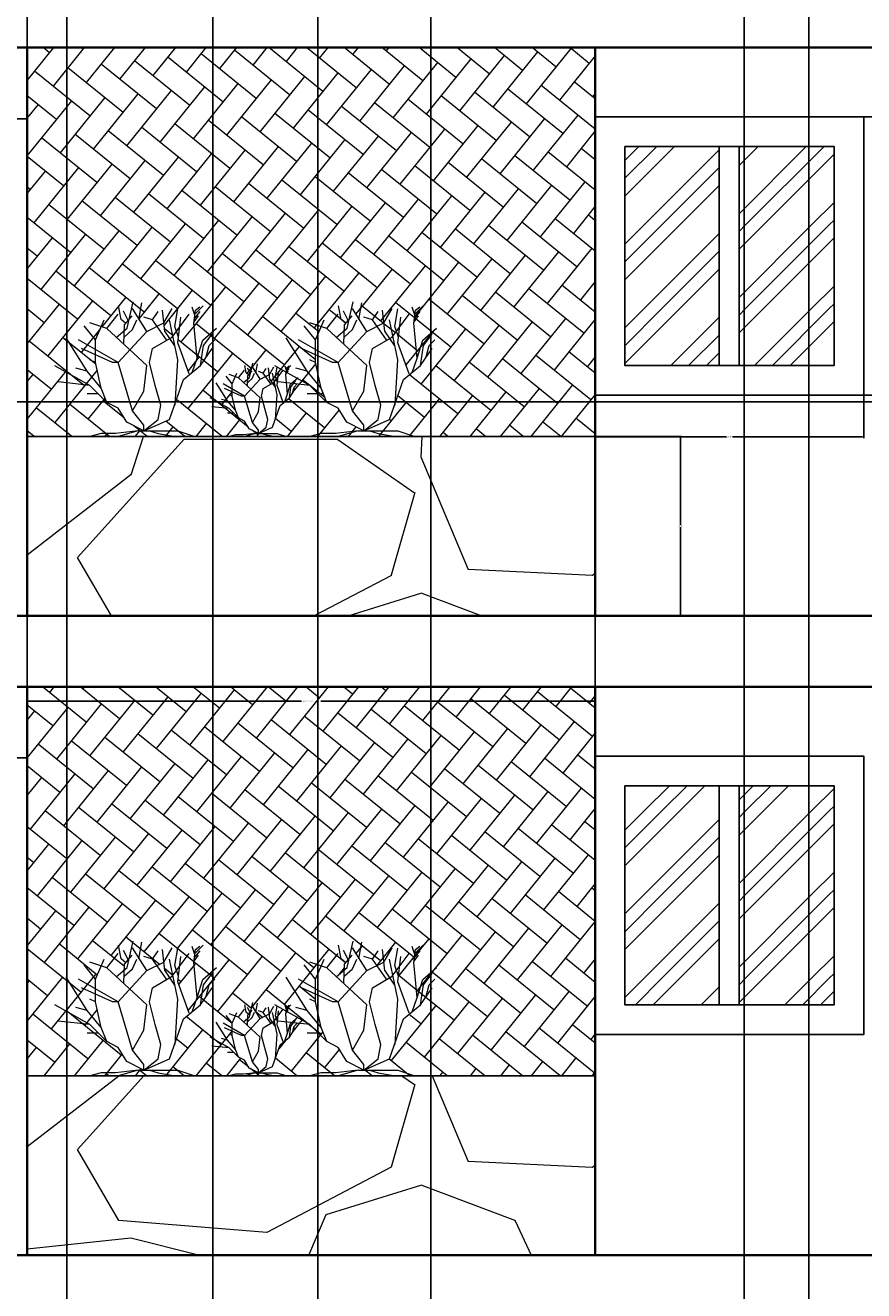
# Model space of a CAD drawing. Units: inches. Extents: x -8 to 554, y -200 to 499.
# Tile 9 of 12: x 216 to 358, y 121 to 335. Entities that reach past the tile are written whole.
import ezdxf

# ---------------------------------------------------------------- set-up
doc = ezdxf.new("R2010")
doc.units = ezdxf.units.IN
doc.header["$MEASUREMENT"] = 0
for name, color, linetype, lineweight in [('A-ANNO-DIMS', 2, 'Continuous', 18), ('A-DOOR', 3, 'Continuous', 25), ('A-FLOR', 7, 'Continuous', 35), ('A-GLAZ', 4, 'Continuous', 25), ('A-GLAZ-PATT', 252, 'Continuous', 13), ('A-WALL', 7, 'Continuous', 35), ('A-WALL-PATT', 252, 'Continuous', 13), ('A-WALL-PRPT', 7, 'Continuous', 25), ('L-PLNT-TREE', 94, 'Continuous', 13)]:
    doc.layers.add(name, color=color, linetype=linetype, lineweight=lineweight)
doc.styles.get("Standard").update_dxf_attribs({"font": 'arial.ttf'})
doc.dimstyles.get("Standard").update_dxf_attribs({"dimtxt": 0.18, "dimasz": 0.18, "dimexe": 0.18, "dimexo": 0.0625, "dimgap": 0.09, "dimtad": 0, "dimtih": 1, "dimtoh": 1, "dimdec": 4, "dimzin": 0, "dimdsep": 46, "dimtxsty": 'Standard', "dimcen": 0.09, "dimadec": 0, "dimazin": 0, "dimtfac": 1, "dimtdec": 4, "dimtofl": 0, "dimtmove": 0, "dimatfit": 3, "dimfxl": 1, "dimtolj": 1, "dimtzin": 0, "dimarcsym": 0})

# ---------------------------------------------------------------- blocks, each defined once
blk = doc.blocks.new('*U2')
for p, q in [((-12.471, 19.775), (-12.898, 22.044)), ((-11.433, 18.289), (-10.457, 22.749)), ((-8.16, 17.76), (-10.56, 21.6)), ((-9.48, 19.775), (-8.992, 22.592)), ((-5.28, 19.2), (-3.84, 21.6)), ((-3.377, 18.602), (-2.888, 21.575)), ((-0.508, 21.888), (-0.081, 20.558)), ((0.041, 20.714), (1.384, 22.044)), ((0.102, 21.34), (0.835, 21.888)), ((-16.8, 16.32), (-15.36, 19.68)), ((-14.88, 18.24), (-12.96, 20.64)), ((-11.677, 19.071), (-12.471, 19.775)), ((-11.28, 19.619), (-12.104, 21.184)), ((-11.921, 18.836), (-10.64, 20.401)), ((-10.579, 18.054), (-9.846, 19.697)), ((-7.2, 19.68), (-8.64, 20.16)), ((-7.2, 19.68), (-6.24, 21.12)), ((-4.8, 16.32), (-7.2, 19.68)), ((-5.086, 17.741), (-5.513, 21.34)), ((-2.88, 12.96), (-4.32, 19.68)), ((-3.84, 16.8), (-0.96, 20.64)), ((-2.88, 15.84), (-2.4, 20.16)), ((-0.203, 19.149), (0.102, 21.34)), ((-0.142, 19.384), (0.59, 20.401)), ((-0.02, 20.01), (0.896, 21.105)), ((-16.8, 16.32), (-18.72, 18.72)), ((-14.88, 18.24), (-17.76, 19.2)), ((-8.16, 12), (-14.88, 18.24)), ((-13.325, 16.724), (-11.433, 18.289)), ((-12.96, 12.48), (-8.16, 17.76)), ((-12.043, 15.628), (-11.921, 18.836)), ((-11.982, 16.802), (-10.579, 18.054)), ((-8.16, 17.76), (-5.28, 19.2)), ((-3.377, 15.315), (-5.086, 17.819)), ((-2.766, 16.802), (-3.377, 18.602)), ((0.346, 13.203), (-0.203, 19.149)), ((1.323, 16.254), (3.642, 18.289)), ((1.44, 15.36), (2.88, 17.28)), ((-18.24, 11.04), (-21.755, 16.655)), ((-12.96, 12.48), (-19.68, 16.32)), ((-16.8, 12.48), (-16.8, 16.32)), ((-7.2, 14.88), (-3.84, 16.8)), ((-0.96, 10.56), (-2.88, 15.84)), ((0.346, 13.203), (1.323, 16.254)), ((0.96, 12), (1.44, 15.36)), ((1.92, 13.44), (2.4, 15.36)), ((2.4, 15.36), (3.36, 16.32)), ((-13.92, 12.48), (-19.2, 14.88)), ((-16.8, 12.48), (-17.76, 12.96)), ((-7.68, 12.48), (-7.2, 14.88)), ((-3.36, 5.28), (-2.88, 12.96)), ((-0.48, 10.8), (0.346, 13.203)), ((0.96, 12), (2.88, 14.88)), ((-17.76, 8.64), (-23.663, 11.961)), ((-18.24, 11.04), (-20.16, 11.52)), ((-15.84, 8.16), (-18.24, 11.04)), ((-15.84, 8.16), (-16.8, 12.48)), ((-12.96, 12.48), (-13.92, 12.48)), ((-10.56, 4.32), (-12.96, 12.48)), ((-8.64, 7.68), (-8.16, 12)), ((-6.72, 8.64), (-7.68, 12.48)), ((-1.92, 9.6), (0.96, 12)), ((-17.76, 8.64), (-23.128, 9.222)), ((-14.88, 5.76), (-17.76, 8.64)), ((-5.76, 5.28), (-6.72, 8.64)), ((-4.32, 2.88), (-1.92, 9.6)), ((-16.32, 7.2), (-18.24, 7.2)), ((-14.88, 5.76), (-15.84, 8.16)), ((-10.56, 4.32), (-8.64, 7.68)), ((-12.96, 4.8), (-14.88, 5.76)), ((-11.52, 2.4), (-12.96, 4.8)), ((-8.64, 1.92), (-10.56, 4.32)), ((-6.24, 2.88), (-5.76, 5.28)), ((-8.64, 0.96), (-11.52, 2.4)), ((-8.64, 0.96), (-4.32, 2.88)), ((-8.64, 0.96), (-6.24, 2.88)), ((-15.84, 0.48), (-17.76, 0)), ((-13.44, 0.48), (-15.84, 0.48)), ((-9.6, 0.96), (-13.44, 0.48)), ((-9.6, 0.96), (-12.96, 0)), ((-9.6, 0.96), (-7.68, 0.96)), ((-8.64, 0.96), (-8.64, 1.92)), ((-8.64, 0.96), (-2.88, 0.96)), ((-7.68, 0.96), (-6.24, 0.48)), ((-6.24, 0.48), (-3.36, 0)), ((-2.88, 0.96), (0, 0))]:
    blk.add_line(p, q)
blk = doc.blocks.new('BALCONY-FRONT-96IN')
blk.add_line((0, 30.31), (96, 30.31))
blk.add_lwpolyline([(0, 30.31), (0, 0), (96, 0), (96, 30.31)])
blk = doc.blocks.new('WINDOW-CASING-TWO-LIGHT')
blk.add_lwpolyline([(0, 47.03), (45.36, 47.03), (45.36, 0), (0, 0)], close=True)
blk = doc.blocks.new('*D20')
at = {"layer": 'A-ANNO-DIMS', "color": 0, "lineweight": -2, "transparency": 16777216}
for p, q in [((216.34, 235.42), (216.34, 220.9)), ((312.34, 235.42), (312.34, 220.9)), ((216.52, 221.08), (262.71, 221.08)), ((312.16, 221.08), (265.97, 221.08))]:
    blk.add_line(p, q, dxfattribs=at)
at = {"layer": 'A-ANNO-DIMS', "color": 0, "transparency": 16777216}
for points in [[(216.52, 221.11), (216.52, 221.05), (216.34, 221.08)], [(312.16, 221.11), (312.16, 221.05), (312.34, 221.08)]]:
    blk.add_solid(points, dxfattribs=at)
at = {"layer": 'Defpoints', "color": 0, "transparency": 16777216}
for p in [(216.34, 235.48), (312.34, 235.48), (312.34, 221.08)]:
    blk.add_point(p, dxfattribs=at)
at = {"layer": 'A-ANNO-DIMS', "color": 0, "transparency": 16777216, "insert": (264.34, 221.08), "char_height": 0.18, "attachment_point": 5}
blk.add_mtext('\\A1;BALCONY FRONT 96 TYP.', dxfattribs=at)
blk = doc.blocks.new('*D21')
at = {"layer": 'A-ANNO-DIMS', "color": 0, "lineweight": -2, "transparency": 16777216}
for p, q in [((312.4, 265.79), (326.92, 265.79)), ((326.74, 265.61), (326.74, 250.82)), ((326.74, 235.66), (326.74, 250.45)), ((312.4, 235.48), (326.92, 235.48))]:
    blk.add_line(p, q, dxfattribs=at)
at = {"layer": 'A-ANNO-DIMS', "color": 0, "transparency": 16777216}
for points in [[(326.71, 265.61), (326.77, 265.61), (326.74, 265.79)], [(326.71, 235.66), (326.77, 235.66), (326.74, 235.48)]]:
    blk.add_solid(points, dxfattribs=at)
at = {"layer": 'Defpoints', "color": 0, "transparency": 16777216}
for p in [(312.34, 265.79), (326.74, 265.79), (312.34, 235.48)]:
    blk.add_point(p, dxfattribs=at)
at = {"layer": 'A-ANNO-DIMS', "color": 0, "transparency": 16777216, "insert": (326.74, 250.64), "char_height": 0.18, "attachment_point": 5}
blk.add_mtext('\\A1;30 TYP.', dxfattribs=at)
blk = doc.blocks.new('*D26')
at = {"layer": 'A-ANNO-DIMS', "color": 0, "lineweight": -2, "transparency": 16777216}
for p, q in [((357.76, 319.79), (364.93, 319.79)), ((364.75, 319.61), (364.75, 296.46)), ((364.75, 272.94), (364.75, 296.09)), ((357.76, 272.76), (364.93, 272.76))]:
    blk.add_line(p, q, dxfattribs=at)
at = {"layer": 'A-ANNO-DIMS', "color": 0, "transparency": 16777216}
for points in [[(364.72, 319.61), (364.78, 319.61), (364.75, 319.79)], [(364.72, 272.94), (364.78, 272.94), (364.75, 272.76)]]:
    blk.add_solid(points, dxfattribs=at)
at = {"layer": 'Defpoints', "color": 0, "transparency": 16777216}
for p in [(357.7, 319.79), (364.75, 319.79), (357.7, 272.76)]:
    blk.add_point(p, dxfattribs=at)
at = {"layer": 'A-ANNO-DIMS', "color": 0, "transparency": 16777216, "insert": (364.75, 296.28), "char_height": 0.18, "attachment_point": 5}
blk.add_mtext('\\A1;TWO-LIGHT CASING 47 TYP.', dxfattribs=at)
blk = doc.blocks.new('*D27')
at = {"layer": 'A-ANNO-DIMS', "color": 0, "lineweight": -2, "transparency": 16777216}
for p, q in [((312.34, 272.7), (312.34, 265.53)), ((357.7, 272.7), (357.7, 265.53)), ((312.52, 265.71), (334.49, 265.71)), ((357.52, 265.71), (335.55, 265.71))]:
    blk.add_line(p, q, dxfattribs=at)
at = {"layer": 'A-ANNO-DIMS', "color": 0, "transparency": 16777216}
for points in [[(312.52, 265.74), (312.52, 265.68), (312.34, 265.71)], [(357.52, 265.74), (357.52, 265.68), (357.7, 265.71)]]:
    blk.add_solid(points, dxfattribs=at)
at = {"layer": 'Defpoints', "color": 0, "transparency": 16777216}
for p in [(312.34, 272.76), (357.7, 272.76), (357.7, 265.71)]:
    blk.add_point(p, dxfattribs=at)
at = {"layer": 'A-ANNO-DIMS', "color": 0, "transparency": 16777216, "insert": (335.02, 265.71), "char_height": 0.18, "attachment_point": 5}
blk.add_mtext('\\A1;45 TYP.', dxfattribs=at)
blk = doc.blocks.new('*D31')
at = {"layer": 'A-ANNO-DIMS', "color": 0, "lineweight": -2, "transparency": 16777216}
for p, q in [((24.34, 127.42), (24.34, -199.97)), ((453.32, -30.73), (453.32, -199.97)), ((24.52, -199.79), (238.54, -199.79)), ((453.14, -199.79), (239.12, -199.79))]:
    blk.add_line(p, q, dxfattribs=at)
at = {"layer": 'A-ANNO-DIMS', "color": 0, "transparency": 16777216}
for points in [[(24.52, -199.76), (24.52, -199.82), (24.34, -199.79)], [(453.14, -199.76), (453.14, -199.82), (453.32, -199.79)]]:
    blk.add_solid(points, dxfattribs=at)
at = {"layer": 'Defpoints', "color": 0, "transparency": 16777216}
for p in [(24.34, 127.48), (453.32, -30.67), (453.32, -199.79)]:
    blk.add_point(p, dxfattribs=at)
at = {"layer": 'A-ANNO-DIMS', "color": 0, "transparency": 16777216, "insert": (238.83, -199.79), "char_height": 0.18, "attachment_point": 5}
blk.add_mtext('\\A1;429', dxfattribs=at)
blk = doc.blocks.new('*D32')
at = {"layer": 'A-ANNO-DIMS', "color": 0, "lineweight": -2, "transparency": 16777216}
for p, q in [((24.34, 223.42), (24.34, -199.97)), ((444.34, 223.42), (444.34, -199.97)), ((24.52, -199.79), (234.05, -199.79)), ((444.16, -199.79), (234.63, -199.79))]:
    blk.add_line(p, q, dxfattribs=at)
at = {"layer": 'A-ANNO-DIMS', "color": 0, "transparency": 16777216}
for points in [[(24.52, -199.76), (24.52, -199.82), (24.34, -199.79)], [(444.16, -199.76), (444.16, -199.82), (444.34, -199.79)]]:
    blk.add_solid(points, dxfattribs=at)
at = {"layer": 'Defpoints', "color": 0, "transparency": 16777216}
for p in [(24.34, 223.48), (444.34, 223.48), (444.34, -199.79)]:
    blk.add_point(p, dxfattribs=at)
at = {"layer": 'A-ANNO-DIMS', "color": 0, "transparency": 16777216, "insert": (234.34, -199.79), "char_height": 0.18, "attachment_point": 5}
blk.add_mtext('\\A1;420', dxfattribs=at)
blk = doc.blocks.new('*D43')
at = {"layer": 'A-ANNO-DIMS', "color": 0, "lineweight": -2, "transparency": 16777216}
for p, q in [((168.34, 319.54), (168.34, 498.99)), ((168.52, 498.81), (192.12, 498.81)), ((216.16, 498.81), (192.56, 498.81)), ((216.34, 319.54), (216.34, 498.99))]:
    blk.add_line(p, q, dxfattribs=at)
at = {"layer": 'A-ANNO-DIMS', "color": 0, "transparency": 16777216}
for points in [[(168.52, 498.84), (168.52, 498.78), (168.34, 498.81)], [(216.16, 498.84), (216.16, 498.78), (216.34, 498.81)]]:
    blk.add_solid(points, dxfattribs=at)
at = {"layer": 'Defpoints', "color": 0, "transparency": 16777216}
for p in [(216.34, 498.81), (168.34, 319.48), (216.34, 319.48)]:
    blk.add_point(p, dxfattribs=at)
at = {"layer": 'A-ANNO-DIMS', "color": 0, "transparency": 16777216, "insert": (192.34, 498.81), "char_height": 0.18, "attachment_point": 5}
blk.add_mtext('\\A1;48', dxfattribs=at)
blk = doc.blocks.new('*D46')
at = {"layer": 'A-ANNO-DIMS', "color": 0, "lineweight": -2, "transparency": 16777216}
for p, q in [((101.04, 271.66), (554.26, 271.66)), ((554.08, 271.48), (554.08, 253.75)), ((554.08, 235.66), (554.08, 253.39)), ((66.27, 235.48), (554.26, 235.48))]:
    blk.add_line(p, q, dxfattribs=at)
at = {"layer": 'A-ANNO-DIMS', "color": 0, "transparency": 16777216}
for points in [[(554.05, 271.48), (554.11, 271.48), (554.08, 271.66)], [(554.05, 235.66), (554.11, 235.66), (554.08, 235.48)]]:
    blk.add_solid(points, dxfattribs=at)
at = {"layer": 'Defpoints', "color": 0, "transparency": 16777216}
for p in [(100.98, 271.66), (66.2, 235.48), (554.08, 235.48)]:
    blk.add_point(p, dxfattribs=at)
at = {"layer": 'A-ANNO-DIMS', "color": 0, "transparency": 16777216, "insert": (554.08, 253.57), "char_height": 0.18, "attachment_point": 5}
blk.add_mtext('\\A1;36.18', dxfattribs=at)
blk = doc.blocks.new('*D47')
at = {"layer": 'A-ANNO-DIMS', "color": 0, "lineweight": -2, "transparency": 16777216}
for p, q in [((357.76, 272.76), (554.26, 272.76)), ((554.08, 272.58), (554.08, 254.3)), ((554.08, 235.66), (554.08, 253.94)), ((312.4, 235.48), (554.26, 235.48))]:
    blk.add_line(p, q, dxfattribs=at)
at = {"layer": 'A-ANNO-DIMS', "color": 0, "transparency": 16777216}
for points in [[(554.05, 272.58), (554.11, 272.58), (554.08, 272.76)], [(554.05, 235.66), (554.11, 235.66), (554.08, 235.48)]]:
    blk.add_solid(points, dxfattribs=at)
at = {"layer": 'Defpoints', "color": 0, "transparency": 16777216}
for p in [(357.7, 272.76), (312.34, 235.48), (554.08, 235.48)]:
    blk.add_point(p, dxfattribs=at)
at = {"layer": 'A-ANNO-DIMS', "color": 0, "transparency": 16777216, "insert": (554.08, 254.12), "char_height": 0.18, "attachment_point": 5}
blk.add_mtext('\\A1;37.28', dxfattribs=at)
blk = doc.blocks.new('*D55')
at = {"layer": 'A-ANNO-DIMS', "color": 0, "lineweight": -2, "transparency": 16777216}
for p, q in [((204.61, -30.61), (204.61, 498.99)), ((204.79, 498.81), (328.57, 498.81)), ((453.14, 498.81), (329.36, 498.81)), ((453.32, -30.61), (453.32, 498.99))]:
    blk.add_line(p, q, dxfattribs=at)
at = {"layer": 'A-ANNO-DIMS', "color": 0, "transparency": 16777216}
for points in [[(204.79, 498.84), (204.79, 498.78), (204.61, 498.81)], [(453.14, 498.84), (453.14, 498.78), (453.32, 498.81)]]:
    blk.add_solid(points, dxfattribs=at)
at = {"layer": 'Defpoints', "color": 0, "transparency": 16777216}
for p in [(453.32, 498.81), (204.61, -30.67), (453.32, -30.67)]:
    blk.add_point(p, dxfattribs=at)
at = {"layer": 'A-ANNO-DIMS', "color": 0, "transparency": 16777216, "insert": (328.96, 498.81), "char_height": 0.18, "attachment_point": 5}
blk.add_mtext('\\A1;248.7', dxfattribs=at)
blk = doc.blocks.new('*D62')
at = {"layer": 'A-ANNO-DIMS', "color": 0, "lineweight": -2, "transparency": 16777216}
for p, q in [((189.3, 7.54), (189.3, 498.99)), ((189.48, 498.81), (263.01, 498.81)), ((337.31, 498.81), (263.78, 498.81)), ((337.49, 7.54), (337.49, 498.99))]:
    blk.add_line(p, q, dxfattribs=at)
at = {"layer": 'A-ANNO-DIMS', "color": 0, "transparency": 16777216}
for points in [[(189.48, 498.84), (189.48, 498.78), (189.3, 498.81)], [(337.31, 498.84), (337.31, 498.78), (337.49, 498.81)]]:
    blk.add_solid(points, dxfattribs=at)
at = {"layer": 'Defpoints', "color": 0, "transparency": 16777216}
for p in [(337.49, 498.81), (189.3, 7.48), (337.49, 7.48)]:
    blk.add_point(p, dxfattribs=at)
at = {"layer": 'A-ANNO-DIMS', "color": 0, "transparency": 16777216, "insert": (263.4, 498.81), "char_height": 0.18, "attachment_point": 5}
blk.add_mtext('\\A1;148.2', dxfattribs=at)
blk = doc.blocks.new('*D63')
at = {"layer": 'A-ANNO-DIMS', "color": 0, "lineweight": -2, "transparency": 16777216}
for p, q in [((337.49, -52.76), (337.49, 498.99)), ((337.67, 498.81), (342.51, 498.81)), ((348.26, 498.81), (343.42, 498.81)), ((348.44, -52.76), (348.44, 498.99))]:
    blk.add_line(p, q, dxfattribs=at)
at = {"layer": 'A-ANNO-DIMS', "color": 0, "transparency": 16777216}
for points in [[(337.67, 498.84), (337.67, 498.78), (337.49, 498.81)], [(348.26, 498.84), (348.26, 498.78), (348.44, 498.81)]]:
    blk.add_solid(points, dxfattribs=at)
at = {"layer": 'Defpoints', "color": 0, "transparency": 16777216}
for p in [(348.44, 498.81), (337.49, -52.82), (348.44, -52.82)]:
    blk.add_point(p, dxfattribs=at)
at = {"layer": 'A-ANNO-DIMS', "color": 0, "transparency": 16777216, "insert": (342.97, 498.81), "char_height": 0.18, "attachment_point": 5}
blk.add_mtext('\\A1;10.946', dxfattribs=at)
blk = doc.blocks.new('*D64')
at = {"layer": 'A-ANNO-DIMS', "color": 0, "lineweight": -2, "transparency": 16777216}
for p, q in [((337.49, 7.54), (337.49, 498.99)), ((337.67, 498.81), (379.02, 498.81)), ((421.13, 498.81), (379.78, 498.81)), ((421.31, 7.54), (421.31, 498.99))]:
    blk.add_line(p, q, dxfattribs=at)
at = {"layer": 'A-ANNO-DIMS', "color": 0, "transparency": 16777216}
for points in [[(337.67, 498.84), (337.67, 498.78), (337.49, 498.81)], [(421.13, 498.84), (421.13, 498.78), (421.31, 498.81)]]:
    blk.add_solid(points, dxfattribs=at)
at = {"layer": 'Defpoints', "color": 0, "transparency": 16777216}
for p in [(421.31, 498.81), (337.49, 7.48), (421.31, 7.48)]:
    blk.add_point(p, dxfattribs=at)
at = {"layer": 'A-ANNO-DIMS', "color": 0, "transparency": 16777216, "insert": (379.4, 498.81), "char_height": 0.18, "attachment_point": 5}
blk.add_mtext('\\A1;83.81', dxfattribs=at)
blk = doc.blocks.new('*D67')
at = {"layer": 'A-ANNO-DIMS', "color": 0, "lineweight": -2, "transparency": 16777216}
for p, q in [((223.01, 427.42), (223.01, -199.97)), ((247.72, 427.42), (247.72, -199.97)), ((223.19, -199.79), (234.9, -199.79)), ((247.54, -199.79), (235.83, -199.79))]:
    blk.add_line(p, q, dxfattribs=at)
at = {"layer": 'A-ANNO-DIMS', "color": 0, "transparency": 16777216}
for points in [[(223.19, -199.76), (223.19, -199.82), (223.01, -199.79)], [(247.54, -199.76), (247.54, -199.82), (247.72, -199.79)]]:
    blk.add_solid(points, dxfattribs=at)
at = {"layer": 'Defpoints', "color": 0, "transparency": 16777216}
for p in [(223.01, 427.48), (247.72, 427.48), (247.72, -199.79)]:
    blk.add_point(p, dxfattribs=at)
at = {"layer": 'A-ANNO-DIMS', "color": 0, "transparency": 16777216, "insert": (235.36, -199.79), "char_height": 0.18, "attachment_point": 5}
blk.add_mtext('\\A1;24.705', dxfattribs=at)
blk = doc.blocks.new('*D68')
at = {"layer": 'A-ANNO-DIMS', "color": 0, "lineweight": -2, "transparency": 16777216}
for p, q in [((247.72, 371.73), (247.72, -199.97)), ((265.46, 371.73), (265.46, -199.97)), ((247.9, -199.79), (256.13, -199.79)), ((265.28, -199.79), (257.04, -199.79))]:
    blk.add_line(p, q, dxfattribs=at)
at = {"layer": 'A-ANNO-DIMS', "color": 0, "transparency": 16777216}
for points in [[(247.9, -199.76), (247.9, -199.82), (247.72, -199.79)], [(265.28, -199.76), (265.28, -199.82), (265.46, -199.79)]]:
    blk.add_solid(points, dxfattribs=at)
at = {"layer": 'Defpoints', "color": 0, "transparency": 16777216}
for p in [(247.72, 371.79), (265.46, 371.79), (265.46, -199.79)]:
    blk.add_point(p, dxfattribs=at)
at = {"layer": 'A-ANNO-DIMS', "color": 0, "transparency": 16777216, "insert": (256.59, -199.79), "char_height": 0.18, "attachment_point": 5}
blk.add_mtext('\\A1;17.744', dxfattribs=at)
blk = doc.blocks.new('*D69')
at = {"layer": 'A-ANNO-DIMS', "color": 0, "lineweight": -2, "transparency": 16777216}
for p, q in [((265.46, 371.73), (265.46, -199.97)), ((284.57, 371.73), (284.57, -199.97)), ((265.64, -199.79), (274.65, -199.79)), ((284.39, -199.79), (275.38, -199.79))]:
    blk.add_line(p, q, dxfattribs=at)
at = {"layer": 'A-ANNO-DIMS', "color": 0, "transparency": 16777216}
for points in [[(265.64, -199.76), (265.64, -199.82), (265.46, -199.79)], [(284.39, -199.76), (284.39, -199.82), (284.57, -199.79)]]:
    blk.add_solid(points, dxfattribs=at)
at = {"layer": 'Defpoints', "color": 0, "transparency": 16777216}
for p in [(265.46, 371.79), (284.57, 371.79), (284.57, -199.79)]:
    blk.add_point(p, dxfattribs=at)
at = {"layer": 'A-ANNO-DIMS', "color": 0, "transparency": 16777216, "insert": (275.01, -199.79), "char_height": 0.18, "attachment_point": 5}
blk.add_mtext('\\A1;19.11', dxfattribs=at)

msp = doc.modelspace()

# ---------------------------------------------------------------- hatches: boundary and pattern name
at = {"layer": 'A-GLAZ-PATT'}
h = msp.add_hatch(dxfattribs=at)
h.set_pattern_fill('GOST_GROUND', color=256)
h.set_pattern_definition([(45, (-117.809, -80.312), (14.14214, 0), [20]), (45, (-114.809, -80.312), (14.14214, 0), [20]), (45, (-111.809, -80.312), (14.14214, 0), [20])])
h.paths.add_polyline_path([(83.5906, 206.2713), (71.2048, 206.2713), (71.2048, 187.4661), (83.5906, 187.4661)])
h.paths.add_polyline_path([(95.9765, 187.4661), (83.5906, 187.4661), (83.5906, 168.661), (95.9765, 168.661)])
h.paths.add_polyline_path([(83.5906, 98.2713), (71.2048, 98.2713), (71.2048, 79.4661), (83.5906, 79.4661)])
h.paths.add_polyline_path([(95.9765, 79.4661), (83.5906, 79.4661), (83.5906, 60.661), (95.9765, 60.661)])
h.paths.add_polyline_path([(333.2924, 98.788), (317.3421, 98.788), (317.3421, 61.7623), (333.2924, 61.7623)])
h.paths.add_polyline_path([(352.699, 98.788), (336.6386, 98.788), (336.6386, 61.7623), (352.699, 61.7623)])
h.paths.add_polyline_path([(333.2924, 206.788), (317.3421, 206.788), (317.3421, 169.7623), (333.2924, 169.7623)])
h.paths.add_polyline_path([(352.699, 206.788), (336.6386, 206.788), (336.6386, 169.7623), (352.699, 169.7623)])
h.paths.add_polyline_path([(333.2924, 314.788), (317.3421, 314.788), (317.3421, 277.7623), (333.2924, 277.7623)])
h.paths.add_polyline_path([(352.699, 314.788), (336.6386, 314.788), (336.6386, 277.7623), (352.699, 277.7623)])
h.paths.add_polyline_path([(95.9765, 295.4661), (83.5906, 295.4661), (83.5906, 276.661), (95.9765, 276.661)])
h.paths.add_polyline_path([(83.5906, 314.2713), (71.2048, 314.2713), (71.2048, 295.4661), (83.5906, 295.4661)])
at = {"layer": 'A-WALL-PATT'}
h = msp.add_hatch(dxfattribs=at)
h.set_pattern_fill('GRAVEL', color=256, scale=100)
h.set_pattern_definition([(228.0128, (-45.809, 19.688), (-800, -900), [13.4536, -1331.909]), (184.9697, (-54.8087, 9.688), (1200, 100), [23.0868, -2285.5925]), (132.5104, (-77.809, 7.688), (1000, -1100), [16.279, -1611.6033]), (267.2737, (-116.8087, -17.312), (100, 2000), [21.0238, -2081.3558]), (292.83365, (-117.8087, -38.312), (-500, 1200), [20.6155, -2040.9373]), (357.2737, (-109.8087, -57.312), (-2000, 100), [21.0238, -2081.3558]), (37.69424, (-88.8087, -58.3118), (-1300, -1000), [27.803, -2752.4849]), (72.2553, (-66.8087, -41.312), (700, 2200), [26.2488, -2598.632]), (121.4296, (-58.8087, -16.312), (-800, 1300), [21.095, -2088.4073]), (175.2364, (-69.809, 1.688), (1100, -100), [24.083, -1180.076]), (222.39744, (-93.8087, 3.6882), (-1200, -1100), [31.1448, -3083.3375]), (138.814, (-17.809, -18.312), (-700, 600), [10.63, -1052.3845]), (171.4692, (-25.8087, -11.312), (1300, -200), [20.2237, -2002.151]), (225, (-45.81, -8.31), (-1e-14, -100), [14.142, -127.279]), (203.1986, (-52.809, 3.688), (500, 200), [7.616, -753.9615]), (291.8014, (-59.809, 0.688), (-100, 300), [10.77, -527.746]), (30.9638, (-55.809, -9.312), (300, 200), [17.493, -565.602]), (161.565, (-40.81, -0.312), (200, -100), [12.649, -303.579]), (16.3895, (-117.8087, 0.688), (1000, 300), [17.72, -1754.2845]), (70.3462, (-100.809, 5.688), (-400, -1100), [14.866, -1471.741]), (293.1986, (-40.809, 19.688), (-200, 500), [15.2315, -746.346]), (343.6105, (-34.8087, 5.688), (-1000, 300), [17.72, -1754.2845]), (339.444, (-117.809, -61.312), (-500, 200), [17.088, -837.3124]), (294.7751, (-101.809, -67.312), (-500, 1100), [14.318, -1417.4643]), (66.8014, (-39.809, -80.312), (200, 500), [15.2315, -746.346]), (17.354, (-33.809, -66.312), (-1300, -400), [16.763, -1659.5424]), (69.444, (-88.809, -80.312), (-200, -500), [8.544, -845.8564]), (101.31, (-45.809, -80.312), (-100, 400), [5.099, -504.803]), (165.9638, (-46.809, -75.312), (300, -100), [20.6155, -391.695]), (186.009, (-66.8087, -70.312), (1000, 100), [19.105, -1891.3923]), (303.69, (-55.81, -18.312), (-100, 200), [14.422, -346.133]), (353.1572, (-47.8087, -30.312), (1700, -200), [25.1794, -2492.7563]), (60.9454, (-22.809, -33.312), (-400, -700), [10.2956, -1019.2674]), (90, (-17.81, -24.31), (-100, 100), [6, -94]), (120.2564, (-68.809, -67.312), (400, -700), [13.8924, -1375.352]), (48.0128, (-75.809, -55.312), (800, 900), [26.907, -1318.455]), (0, (-57.81, -35.31), (100, 100), [26, -74]), (325.3048, (-31.809, -35.312), (1000, -700), [15.8114, -1565.3274]), (254.0546, (-18.809, -44.312), (-100, -400), [14.56, -713.451]), (207.646, (-22.8087, -58.312), (-1900, -1000), [23.7065, -2346.9474]), (175.4261, (-43.8087, -69.312), (-1300, 100), [25.08, -2482.9073])])
h.paths.add_polyline_path([(48.6882, -52.5186), (24.3421, -52.5186), (24.3421, -112.5186), (48.6882, -112.5186)])
h.paths.add_polyline_path([(212.2282, -52.5186), (140.2282, -52.5186), (128.2282, -52.5186), (128.2282, -112.5186), (140.2282, -112.5186), (140.2282, -64.9665), (202.9211, -64.9665), (202.9211, -112.5186), (212.2282, -112.5186)])
h.paths.add_polyline_path([(312.3421, 49.7921), (216.3421, 49.7921), (216.3421, 19.4814), (312.3421, 19.4814)])
h.paths.add_polyline_path([(312.3421, 157.7921), (216.3421, 157.7921), (216.3421, 127.4814), (312.3421, 127.4814)])
h.paths.add_polyline_path([(312.3421, 265.7921), (216.3421, 265.7921), (216.3421, 235.4814), (312.3421, 235.4814)])
h.paths.add_polyline_path([(432.5174, 371.7921), (215.6778, 371.7921), (215.6778, 368.5162), (215.6778, 357.6367), (35.7874, 357.6367), (35.7874, 360.9127), (35.7874, 371.7921), (24.3421, 371.7921), (24.3421, 343.4814), (35.7874, 343.4814), (432.5174, 343.4814)])
at = {"layer": 'A-WALL-PATT', "transparency": 33554569}
h = msp.add_hatch(dxfattribs=at)
h.set_pattern_fill('AR-HBONE', color=256, angle=96)
h.set_pattern_definition([(141, (-117.8087, -80.312), (-5.625865, -0.591302), [12, -4]), (231, (-120.9173, -77.7945), (-5.625865, -0.591302), [12, -4])])
h.paths.add_polyline_path([(312.3421, 115.4814), (216.3421, 115.4814), (216.3421, 49.7921), (250.4667, 49.7921), (251.5112, 50.0532), (252.8169, 50.0532), (255.3238, 50.3666), (253.8614, 51.0978), (253.078, 52.4035), (252.0335, 52.9257), (251.5112, 54.2314), (250.9889, 56.5816), (250.9889, 58.6707), (251.5112, 59.8894), (252.0335, 59.7153), (253.4528, 61.4895), (253.992, 60.4655), (254.0945, 60.5908), (253.9087, 59.7419), (253.623, 59.5055), (253.5764, 58.2825), (256.1145, 55.9258), (256.4728, 54.4925), (256.995, 52.6646), (256.632, 50.8494), (255.6521, 50.4139), (255.9505, 50.3144), (258.5619, 50.3144), (312.3421, 49.7921)])
h.paths.add_polyline_path([(260.0854, 60.6921), (260.1153, 60.6752), (260.163, 60.7322), (260.1127, 60.8887)], flags=16)
h.paths.add_polyline_path([(270.7709, 69.6415), (271.1925, 71.568), (273.7025, 67.5521), (276.5825, 68.9921), (276.5999, 69.0212), (276.7653, 67.6275), (277.6264, 66.3658), (278.0225, 66.5921), (279.2746, 68.2617), (278.9825, 65.6321), (280.9471, 60.2293), (281.3825, 60.5921), (282.2085, 62.9951), (281.6472, 69.0743), (281.6854, 69.1274), (281.8332, 70.189), (281.7729, 70.3768), (281.8731, 70.4761), (281.6595, 68.9411), (282.2085, 62.9951), (281.3825, 60.5921), (279.9425, 59.3921), (277.5425, 52.6721), (273.2225, 50.7521), (270.3425, 52.1921), (268.9025, 54.5921), (266.9825, 55.5521), (264.1025, 58.4321), (261.9512, 58.6653), (261.4344, 58.1484), (261.1732, 57.1039), (260.6509, 56.3205), (259.0841, 55.0148), (258.3126, 52.8545), (258.5619, 56.8428), (258.2854, 58.1328), (257.8241, 58.8087), (257.5362, 58.6442), (256.624, 59.9214), (257.2562, 60.2375), (257.2657, 60.2534), (257.3556, 59.4952), (257.8241, 58.8087), (258.0396, 58.9319), (258.7208, 59.8402), (258.6303, 59.0254), (264.1025, 58.4321), (266.9825, 55.5521), (266.0225, 57.9521), (265.0625, 62.2721), (265.0625, 66.1121), (266.0225, 68.3521), (266.9825, 68.0321), (268.5785, 66.5501), (269.9041, 67.6466), (269.9415, 68.6281)], flags=16)
h.paths.add_polyline_path([(244.6939, 70.4761), (244.4802, 68.9411), (245.0292, 62.9951), (244.2032, 60.5921), (242.7632, 59.3921), (240.3632, 52.6721), (236.0432, 50.7521), (233.1632, 52.1921), (231.7232, 54.5921), (229.8032, 55.5521), (228.8432, 57.9521), (227.8832, 62.2721), (227.8832, 66.1121), (228.8432, 68.3521), (229.8032, 68.0321), (231.3992, 66.5501), (232.7249, 67.6466), (232.7622, 68.6281), (233.5916, 69.6415), (234.0132, 71.568), (236.5232, 67.5521), (239.4032, 68.9921), (239.4206, 69.0212), (239.586, 67.6275), (240.4471, 66.3658), (240.8432, 66.5921), (242.0954, 68.2617), (241.8032, 65.6321), (243.7678, 60.2293), (244.2032, 60.5921), (245.0292, 62.9951), (244.4679, 69.0743), (244.5061, 69.1274), (244.6539, 70.189), (244.5936, 70.3768)], flags=16)
h.paths.add_polyline_path([(312.3421, 223.4814), (216.3421, 223.4814), (216.3421, 157.7921), (312.3421, 157.7921)])
h.paths.add_polyline_path([(260.0854, 168.6921), (260.1153, 168.6752), (260.163, 168.7322), (260.1127, 168.8887)], flags=16)
h.paths.add_polyline_path([(271.1925, 179.568), (273.7025, 175.5521), (276.5825, 176.9921), (276.5999, 177.0212), (276.7653, 175.6275), (277.6264, 174.3658), (278.0225, 174.5921), (279.2746, 176.2617), (278.9825, 173.6321), (280.9471, 168.2293), (281.3825, 168.5921), (282.2085, 170.9951), (281.6472, 177.0743), (281.6854, 177.1274), (281.8332, 178.189), (281.7729, 178.3768), (281.8731, 178.4761), (281.6595, 176.9411), (282.2085, 170.9951), (281.3825, 168.5921), (279.9425, 167.3921), (277.5425, 160.6721), (273.2225, 158.7521), (270.3425, 160.1921), (268.9025, 162.5921), (266.9825, 163.5521), (264.1025, 166.4321), (261.9512, 166.6653), (261.4344, 166.1484), (261.1732, 165.1039), (260.6509, 164.3205), (259.0841, 163.0148), (257.7785, 159.3589), (255.6521, 158.4139), (255.9505, 158.3144), (255.4282, 158.3144), (253.8614, 159.0978), (253.078, 160.4035), (252.0335, 160.9257), (251.5112, 162.2314), (250.9889, 164.5816), (250.9889, 166.6707), (251.5112, 167.8894), (252.0335, 167.7153), (253.2217, 169.2005), (253.344, 168.5504), (253.7597, 168.1818), (254.0945, 168.5908), (254.3239, 169.6389), (255.6894, 167.4541), (257.2562, 168.2375), (257.2657, 168.2534), (257.3556, 167.4952), (257.8241, 166.8087), (258.0396, 166.9319), (258.7208, 167.8402), (258.6303, 167.0254), (264.1025, 166.4321), (266.9825, 163.5521), (266.0225, 165.9521), (265.0625, 170.2721), (265.0625, 174.1121), (266.0225, 176.3521), (266.9825, 176.0321), (268.5785, 174.5501), (269.9041, 175.6466), (269.9415, 176.6281), (270.7709, 177.6415)], flags=16)
h.paths.add_polyline_path([(253.5764, 166.2825), (255.6894, 164.3205), (255.4282, 161.9703), (254.3837, 160.1423), (253.078, 164.5816), (254.1446, 165.7549), (252.9018, 166.909), (253.623, 167.5055)], flags=0)
h.paths.add_polyline_path([(245.0292, 170.9951), (244.2032, 168.5921), (242.7632, 167.3921), (240.3632, 160.6721), (236.0432, 158.7521), (233.1632, 160.1921), (231.7232, 162.5921), (229.8032, 163.5521), (228.8432, 165.9521), (227.8832, 170.2721), (227.8832, 174.1121), (228.8432, 176.3521), (229.8032, 176.0321), (231.3992, 174.5501), (232.7249, 175.6466), (232.7622, 176.6281), (233.5916, 177.6415), (234.0132, 179.568), (236.5232, 175.5521), (239.4032, 176.9921), (239.4206, 177.0212), (239.586, 175.6275), (240.4471, 174.3658), (240.8432, 174.5921), (242.0954, 176.2617), (241.8032, 173.6321), (243.7678, 168.2293), (244.2032, 168.5921), (245.0292, 170.9951), (244.4679, 177.0743), (244.5061, 177.1274), (244.6539, 178.189), (244.5936, 178.3768), (244.6939, 178.4761), (244.4802, 176.9411)], flags=16)
h.paths.add_polyline_path([(312.3421, 331.4814), (216.3421, 331.4814), (216.3421, 265.7921), (312.3421, 265.7921)])
h.paths.add_polyline_path([(260.0854, 276.6921), (260.1153, 276.6752), (260.163, 276.7322), (260.1127, 276.8887)], flags=16)
h.paths.add_polyline_path([(281.8731, 286.4761), (281.6595, 284.9411), (282.2085, 278.9951), (281.3825, 276.5921), (279.9425, 275.3921), (277.5425, 268.6721), (273.2225, 266.7521), (270.3425, 268.1921), (268.9025, 270.5921), (266.9825, 271.5521), (264.1025, 274.4321), (261.9512, 274.6653), (261.4344, 274.1484), (261.1732, 273.1039), (260.6509, 272.3205), (259.0841, 271.0148), (257.7785, 267.3589), (255.6521, 266.4139), (255.9505, 266.3144), (255.4282, 266.3144), (253.8614, 267.0978), (253.078, 268.4035), (252.0335, 268.9257), (251.5112, 270.2314), (250.9889, 272.5816), (250.9889, 274.6707), (251.5112, 275.8894), (252.0335, 275.7153), (253.2217, 277.2005), (253.344, 276.5504), (253.7597, 276.1818), (254.0945, 276.5908), (254.3239, 277.6389), (255.6894, 275.4541), (257.2562, 276.2375), (257.2657, 276.2534), (257.3556, 275.4952), (257.8241, 274.8087), (258.0396, 274.9319), (258.7208, 275.8402), (258.6303, 275.0254), (264.1025, 274.4321), (266.9825, 271.5521), (266.0225, 273.9521), (265.0625, 278.2721), (265.0625, 282.1121), (266.0225, 284.3521), (266.9825, 284.0321), (268.5785, 282.5501), (269.9041, 283.6466), (269.9415, 284.6281), (270.7709, 285.6415), (271.1925, 287.568), (273.7025, 283.5521), (276.5825, 284.9921), (276.5999, 285.0212), (276.7653, 283.6275), (277.6264, 282.3658), (278.0225, 282.5921), (279.2746, 284.2617), (278.9825, 281.6321), (280.9471, 276.2293), (281.3825, 276.5921), (282.2085, 278.9951), (281.6472, 285.0743), (281.6854, 285.1274), (281.8332, 286.189), (281.7729, 286.3768)], flags=16)
h.paths.add_polyline_path([(255.6894, 272.3205), (255.4282, 269.9703), (254.3837, 268.1423), (253.078, 272.5816), (254.1446, 273.7549), (252.9018, 274.909), (253.623, 275.5055), (253.5764, 274.2825)], flags=0)
h.paths.add_polyline_path([(245.0292, 278.9951), (244.2032, 276.5921), (242.7632, 275.3921), (240.3632, 268.6721), (236.0432, 266.7521), (233.1632, 268.1921), (231.7232, 270.5921), (229.8032, 271.5521), (228.8432, 273.9521), (227.8832, 278.2721), (227.8832, 282.1121), (228.8432, 284.3521), (229.8032, 284.0321), (231.3992, 282.5501), (232.7249, 283.6466), (232.7622, 284.6281), (233.5916, 285.6415), (234.0132, 287.568), (236.5232, 283.5521), (239.4032, 284.9921), (239.4206, 285.0212), (239.586, 283.6275), (240.4471, 282.3658), (240.8432, 282.5921), (242.0954, 284.2617), (241.8032, 281.6321), (243.7678, 276.2293), (244.2032, 276.5921), (245.0292, 278.9951), (244.4679, 285.0743), (244.5061, 285.1274), (244.6539, 286.189), (244.5936, 286.3768), (244.6939, 286.4761), (244.4802, 284.9411)], flags=16)

# ---------------------------------------------------------------- linework, layer by layer
at = {"layer": 'A-DOOR'}
for points in [[(216.3421, 235.4814), (168.3421, 235.4814), (168.3421, 319.4814), (216.3421, 319.4814)], [(216.3421, 127.4814), (168.3421, 127.4814), (168.3421, 211.4814), (216.3421, 211.4814)]]:
    msp.add_lwpolyline(points, close=True, dxfattribs=at)
at = {"layer": 'A-FLOR'}
for p, q in [((444.3421, 331.4814), (36.3421, 331.4814)), ((444.3421, 235.4814), (24.3421, 235.4814)), ((36.3421, 235.4814), (444.3421, 235.4814)), ((24.3421, 223.4814), (444.3421, 223.4814)), ((444.3421, 223.4814), (36.3421, 223.4814)), ((432.5174, 127.4814), (24.3421, 127.4814)), ((36.3421, 127.4814), (432.5174, 127.4814))]:
    msp.add_line(p, q, dxfattribs=at)
at = {"layer": 'A-GLAZ'}
for points in [[(317.3421, 314.788), (352.699, 314.788), (352.699, 277.7623), (317.3421, 277.7623)], [(333.2924, 314.788), (336.6386, 314.788), (336.6386, 277.7623), (333.2924, 277.7623)], [(317.3421, 206.788), (352.699, 206.788), (352.699, 169.7623), (317.3421, 169.7623)], [(333.2924, 206.788), (336.6386, 206.788), (336.6386, 169.7623), (333.2924, 169.7623)]]:
    msp.add_lwpolyline(points, close=True, dxfattribs=at)
at = {"layer": 'A-WALL'}
for p, q in [((216.3421, 235.4814), (216.3421, 331.4814)), ((312.3421, 235.4814), (312.3421, 331.4814)), ((216.3421, 127.4814), (216.3421, 223.4814)), ((312.3421, 127.4814), (312.3421, 223.4814))]:
    msp.add_line(p, q, dxfattribs=at)

# ---------------------------------------------------------------- block references
at = {"layer": 'A-GLAZ'}
for p in [(312.3421, 272.7623), (312.3421, 164.7623)]:
    msp.add_blockref('WINDOW-CASING-TWO-LIGHT', p, dxfattribs=at)
at = {"layer": 'A-WALL-PRPT'}
for p in [(216.3421, 235.4814), (216.3421, 127.4814)]:
    msp.add_blockref('BALCONY-FRONT-96IN', p, dxfattribs=at)
at = {"layer": 'L-PLNT-TREE'}
for p in [(244.6832, 265.7921), (281.8625, 265.7921), (244.6832, 157.7921), (281.8625, 157.7921)]:
    msp.add_blockref('*U2', p, dxfattribs=at)
at = {"layer": 'L-PLNT-TREE', "xscale": 0.5440329233585479, "yscale": 0.5440329233585479, "zscale": 0.5440329233585479}
for p in [(260.1287, 265.7921), (260.1287, 157.7921)]:
    msp.add_blockref('*U2', p, dxfattribs=at)

# ---------------------------------------------------------------- dimensions: what is measured, and where the dimension line sits
at = {"layer": 'A-ANNO-DIMS'}
for base, p1, p2, override, picture, middle in [((216.3421, 498.8091), (168.3421, 319.4814), (216.3421, 319.4814), {"dimdec": 0, "dimlfac": 1, "dimrnd": 0, "dimzin": 0, "dimdsep": 46, "dimlunit": 2}, '*D43', (192.3421, 498.8091)), ((337.4923, 498.8091), (189.3049, 7.4814), (337.4923, 7.4814), {"dimdec": 1, "dimlfac": 1, "dimrnd": 0, "dimzin": 0, "dimdsep": 46, "dimlunit": 2}, '*D62', (263.3986, 498.8091)), ((453.3222, 498.8091), (204.6055, -30.6677), (453.3222, -30.6677), {"dimdec": 1, "dimlfac": 1, "dimrnd": 0, "dimzin": 0, "dimdsep": 46, "dimlunit": 2}, '*D55', (328.9639, 498.8091)), ((348.4381, 498.8091), (337.4923, -52.8231), (348.4381, -52.8231), {"dimdec": 3, "dimlfac": 1, "dimrnd": 0, "dimzin": 0, "dimdsep": 46, "dimlunit": 2}, '*D63', (342.9652, 498.8091)), ((421.3053, 498.8091), (337.4923, 7.4814), (421.3053, 7.4814), {"dimdec": 2, "dimlfac": 1, "dimrnd": 0, "dimzin": 0, "dimdsep": 46, "dimlunit": 2}, '*D64', (379.3988, 498.8091)), ((247.71587, -199.79119), (223.01039, 427.48136), (247.71587, 427.48136), {"dimdec": 3, "dimlfac": 1, "dimrnd": 0, "dimzin": 0, "dimdsep": 46, "dimlunit": 2}, '*D67', (235.36313, -199.79119)), ((265.4598, -199.7912), (247.7159, 371.7921), (265.4598, 371.7921), {"dimdec": 3, "dimlfac": 1, "dimrnd": 0, "dimzin": 0, "dimdsep": 46, "dimlunit": 2}, '*D68', (256.5878, -199.7912)), ((284.5686, -199.7912), (265.4598, 371.7921), (284.5686, 371.7921), {"dimdec": 2, "dimlfac": 1, "dimrnd": 0, "dimzin": 0, "dimdsep": 46, "dimlunit": 2}, '*D69', (275.0142, -199.7912)), ((444.3421, -199.7912), (24.3421, 223.4814), (444.3421, 223.4814), {"dimdec": 0, "dimlfac": 1, "dimrnd": 0, "dimzin": 0, "dimdsep": 46, "dimlunit": 2}, '*D32', (234.3421, -199.7912)), ((453.3222, -199.7912), (24.3421, 127.4814), (453.3222, -30.6677), {"dimdec": 0, "dimlfac": 1, "dimrnd": 0, "dimzin": 0, "dimdsep": 46, "dimlunit": 2}, '*D31', (238.8321, -199.7912))]:
    dim = msp.add_linear_dim(base=base, p1=p1, p2=p2, dimstyle='Standard', override=override, dxfattribs=at)
    dim.commit()
    dim.dimension.update_dxf_attribs({"geometry": picture, "text_midpoint": middle})
for base, p1, p2, text, picture, middle in [((364.7529, 319.788), (357.699, 272.7623), (357.699, 319.788), 'TWO-LIGHT CASING <> TYP.', '*D26', (364.7529, 296.2752)), ((326.7421, 265.7921), (312.3421, 235.4814), (312.3421, 265.7921), '<> TYP.', '*D21', (326.7421, 250.6367))]:
    dim = msp.add_linear_dim(base=base, p1=p1, p2=p2, angle=90, text=text, dimstyle='Standard', override={"dimdec": 0, "dimlfac": 1, "dimrnd": 0, "dimzin": 0, "dimdsep": 46, "dimlunit": 2}, dxfattribs=at)
    dim.commit()
    dim.dimension.update_dxf_attribs({"geometry": picture, "text_midpoint": middle})
for p1, p2, picture, middle in [((100.9765, 271.661), (66.2048, 235.4814), '*D46', (554.0833, 253.5712)), ((357.699, 272.7623), (312.3421, 235.4814), '*D47', (554.0833, 254.1218))]:
    dim = msp.add_linear_dim(base=(554.0833, 235.4814), p1=p1, p2=p2, angle=90, dimstyle='Standard', override={"dimdec": 2, "dimlfac": 1, "dimrnd": 0, "dimzin": 0, "dimdsep": 46, "dimlunit": 2}, dxfattribs=at)
    dim.commit()
    dim.dimension.update_dxf_attribs({"geometry": picture, "text_midpoint": middle})
for base, p1, p2, text, picture, middle in [((357.699, 265.7085), (312.3421, 272.7623), (357.699, 272.7623), '<> TYP.', '*D27', (335.0206, 265.7085)), ((312.3421, 221.0814), (216.3421, 235.4814), (312.3421, 235.4814), 'BALCONY FRONT <> TYP.', '*D20', (264.3421, 221.0814))]:
    dim = msp.add_linear_dim(base=base, p1=p1, p2=p2, text=text, dimstyle='Standard', override={"dimdec": 0, "dimlfac": 1, "dimrnd": 0, "dimzin": 0, "dimdsep": 46, "dimlunit": 2}, dxfattribs=at)
    dim.commit()
    dim.dimension.update_dxf_attribs({"geometry": picture, "text_midpoint": middle})

doc.saveas('drawing.dxf')
